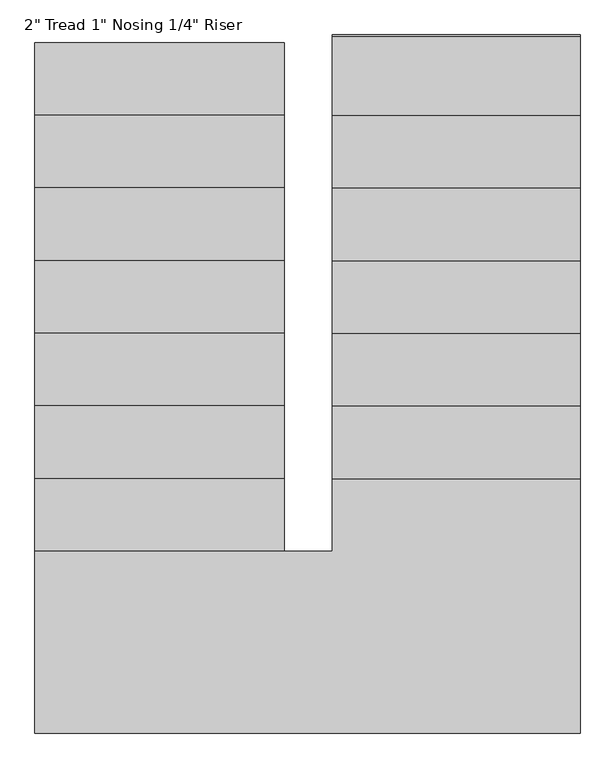
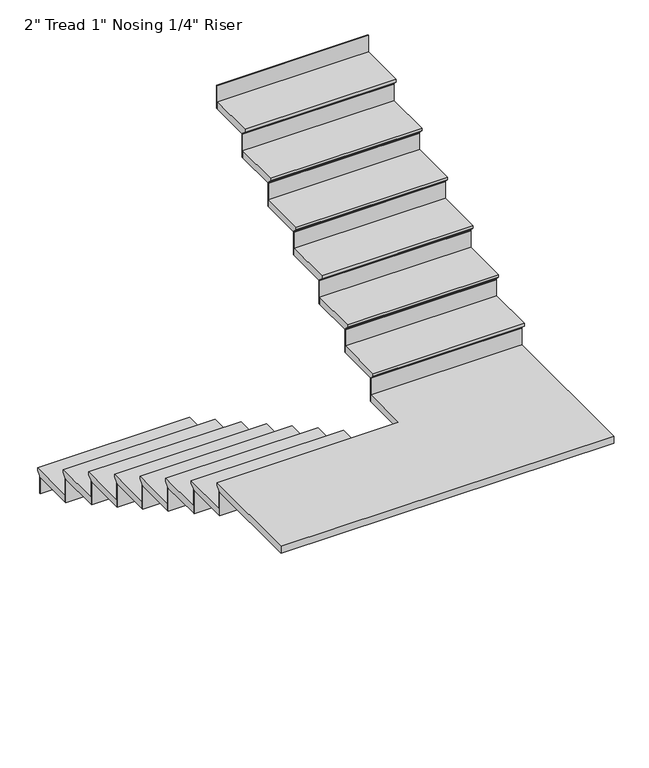
"""IFC4 building model written with IfcOpenShell, lengths in millimetres: stair flight geometry."""

from ifc_helpers import new_model, si_unit, origin, place, context, project, spatial, faceted_brep, source, transform, mapped, element, save


def stair_flight_d5b1d6b9(model_context):
    return source(origin(), model_context, "Body", "Brep", [
        faceted_brep([(-4232.280864, -3571.6080018, 3198.2833333), (-4232.280864, -3571.6080018, 3217.3333333), (-3187.6083919, -3571.6080018, 3217.3333333), (-3187.6083919, -3571.6080018, 3198.2833333), (-4232.280864, -3597.0080018, 3172.8833333), (-3187.6083919, -3597.0080018, 3172.8833333), (-4232.280864, -3901.8080018, 3217.3333333), (-3187.6083919, -3901.8080018, 3217.3333333), (-3187.6083919, -3597.0080018, 3166.5333333), (-3187.6083919, -3901.8080018, 3166.5333333), (-4232.280864, -3901.8080018, 3166.5333333), (-4232.280864, -3597.0080018, 3166.5333333)], [[[0, 1, 2, 3]], [[4, 0, 3, 5]], [[2, 1, 6, 7]], [[8, 9, 10, 11]], [[2, 7, 9, 8, 5, 3]], [[8, 11, 4, 5]], [[6, 1, 0, 4, 11, 10]], [[7, 6, 10, 9]]]),
        faceted_brep([(-4232.280864, -3597.0080018, 3166.5333333), (-4232.280864, -3597.0080018, 3048.0), (-4232.280864, -3603.3580018, 3048.0), (-4232.280864, -3603.3580018, 3166.5333333), (-3187.6083919, -3597.0080018, 3166.5333333), (-3187.6083919, -3603.3580018, 3166.5333333), (-3187.6083919, -3603.3580018, 3048.0), (-3187.6083919, -3597.0080018, 3048.0)], [[[0, 1, 2, 3]], [[4, 5, 6, 7]], [[1, 0, 4, 7]], [[2, 1, 7, 6]], [[3, 2, 6, 5]], [[0, 3, 5, 4]]]),
        faceted_brep([(-4232.280864, -3901.8080018, 3335.8666667), (-4232.280864, -3901.8080018, 3166.5333333), (-4232.280864, -3908.1580018, 3166.5333333), (-4232.280864, -3908.1580018, 3335.8666667), (-3187.6083919, -3901.8080018, 3335.8666667), (-3187.6083919, -3908.1580018, 3335.8666667), (-3187.6083919, -3908.1580018, 3166.5333333), (-3187.6083919, -3901.8080018, 3166.5333333)], [[[0, 1, 2, 3]], [[4, 5, 6, 7]], [[1, 0, 4, 7]], [[2, 1, 7, 6]], [[3, 2, 6, 5]], [[0, 3, 5, 4]]]),
        faceted_brep([(-3187.6083919, -3876.4080018, 3386.6666667), (-4232.280864, -3876.4080018, 3386.6666667), (-4232.280864, -4206.6080018, 3386.6666667), (-3187.6083919, -4206.6080018, 3386.6666667), (-3187.6083919, -3901.8080018, 3335.8666667), (-3187.6083919, -4206.6080018, 3335.8666667), (-4232.280864, -4206.6080018, 3335.8666667), (-4232.280864, -3901.8080018, 3335.8666667), (-3187.6083919, -3901.8080018, 3342.2166667), (-3187.6083919, -3876.4080018, 3367.6166667), (-4232.280864, -3901.8080018, 3342.2166667), (-4232.280864, -3876.4080018, 3367.6166667)], [[[0, 1, 2, 3]], [[4, 5, 6, 7]], [[0, 3, 5, 4, 8, 9]], [[4, 7, 10, 8]], [[2, 1, 11, 10, 7, 6]], [[3, 2, 6, 5]], [[11, 1, 0, 9]], [[10, 11, 9, 8]]]),
        faceted_brep([(-4232.280864, -4206.6080018, 3505.2), (-4232.280864, -4206.6080018, 3335.8666667), (-4232.280864, -4212.9580018, 3335.8666667), (-4232.280864, -4212.9580018, 3505.2), (-3187.6083919, -4206.6080018, 3505.2), (-3187.6083919, -4212.9580018, 3505.2), (-3187.6083919, -4212.9580018, 3335.8666667), (-3187.6083919, -4206.6080018, 3335.8666667)], [[[0, 1, 2, 3]], [[4, 5, 6, 7]], [[1, 0, 4, 7]], [[2, 1, 7, 6]], [[3, 2, 6, 5]], [[0, 3, 5, 4]]]),
        faceted_brep([(-3187.6083919, -4181.2080018, 3556.0), (-4232.280864, -4181.2080018, 3556.0), (-4232.280864, -4511.4080018, 3556.0), (-3187.6083919, -4511.4080018, 3556.0), (-3187.6083919, -4206.6080018, 3505.2), (-3187.6083919, -4511.4080018, 3505.2), (-4232.280864, -4511.4080018, 3505.2), (-4232.280864, -4206.6080018, 3505.2), (-3187.6083919, -4206.6080018, 3511.55), (-3187.6083919, -4181.2080018, 3536.95), (-4232.280864, -4206.6080018, 3511.55), (-4232.280864, -4181.2080018, 3536.95)], [[[0, 1, 2, 3]], [[4, 5, 6, 7]], [[0, 3, 5, 4, 8, 9]], [[4, 7, 10, 8]], [[2, 1, 11, 10, 7, 6]], [[3, 2, 6, 5]], [[11, 1, 0, 9]], [[10, 11, 9, 8]]]),
        faceted_brep([(-4232.280864, -4511.4080018, 3674.5333333), (-4232.280864, -4511.4080018, 3505.2), (-4232.280864, -4517.7580018, 3505.2), (-4232.280864, -4517.7580018, 3674.5333333), (-3187.6083919, -4511.4080018, 3674.5333333), (-3187.6083919, -4517.7580018, 3674.5333333), (-3187.6083919, -4517.7580018, 3505.2), (-3187.6083919, -4511.4080018, 3505.2)], [[[0, 1, 2, 3]], [[4, 5, 6, 7]], [[1, 0, 4, 7]], [[2, 1, 7, 6]], [[3, 2, 6, 5]], [[0, 3, 5, 4]]]),
        faceted_brep([(-3187.6083919, -4486.0080018, 3725.3333333), (-4232.280864, -4486.0080018, 3725.3333333), (-4232.280864, -4816.2080018, 3725.3333333), (-3187.6083919, -4816.2080018, 3725.3333333), (-3187.6083919, -4511.4080018, 3674.5333333), (-3187.6083919, -4816.2080018, 3674.5333333), (-4232.280864, -4816.2080018, 3674.5333333), (-4232.280864, -4511.4080018, 3674.5333333), (-3187.6083919, -4511.4080018, 3680.8833333), (-3187.6083919, -4486.0080018, 3706.2833333), (-4232.280864, -4511.4080018, 3680.8833333), (-4232.280864, -4486.0080018, 3706.2833333)], [[[0, 1, 2, 3]], [[4, 5, 6, 7]], [[0, 3, 5, 4, 8, 9]], [[4, 7, 10, 8]], [[2, 1, 11, 10, 7, 6]], [[3, 2, 6, 5]], [[11, 1, 0, 9]], [[10, 11, 9, 8]]]),
        faceted_brep([(-4232.280864, -4816.2080018, 3843.8666667), (-4232.280864, -4816.2080018, 3674.5333333), (-4232.280864, -4822.5580018, 3674.5333333), (-4232.280864, -4822.5580018, 3843.8666667), (-3187.6083919, -4816.2080018, 3843.8666667), (-3187.6083919, -4822.5580018, 3843.8666667), (-3187.6083919, -4822.5580018, 3674.5333333), (-3187.6083919, -4816.2080018, 3674.5333333)], [[[0, 1, 2, 3]], [[4, 5, 6, 7]], [[1, 0, 4, 7]], [[2, 1, 7, 6]], [[3, 2, 6, 5]], [[0, 3, 5, 4]]]),
        faceted_brep([(-3187.6083919, -4790.8080018, 3894.6666667), (-4232.280864, -4790.8080018, 3894.6666667), (-4232.280864, -5121.0080018, 3894.6666667), (-3187.6083919, -5121.0080018, 3894.6666667), (-3187.6083919, -4816.2080018, 3843.8666667), (-3187.6083919, -5121.0080018, 3843.8666667), (-4232.280864, -5121.0080018, 3843.8666667), (-4232.280864, -4816.2080018, 3843.8666667), (-3187.6083919, -4816.2080018, 3850.2166667), (-3187.6083919, -4790.8080018, 3875.6166667), (-4232.280864, -4816.2080018, 3850.2166667), (-4232.280864, -4790.8080018, 3875.6166667)], [[[0, 1, 2, 3]], [[4, 5, 6, 7]], [[0, 3, 5, 4, 8, 9]], [[4, 7, 10, 8]], [[2, 1, 11, 10, 7, 6]], [[3, 2, 6, 5]], [[11, 1, 0, 9]], [[10, 11, 9, 8]]]),
        faceted_brep([(-4232.280864, -5121.0080018, 4013.2), (-4232.280864, -5121.0080018, 3843.8666667), (-4232.280864, -5127.3580018, 3843.8666667), (-4232.280864, -5127.3580018, 4013.2), (-3187.6083919, -5121.0080018, 4013.2), (-3187.6083919, -5127.3580018, 4013.2), (-3187.6083919, -5127.3580018, 3843.8666667), (-3187.6083919, -5121.0080018, 3843.8666667)], [[[0, 1, 2, 3]], [[4, 5, 6, 7]], [[1, 0, 4, 7]], [[2, 1, 7, 6]], [[3, 2, 6, 5]], [[0, 3, 5, 4]]]),
        faceted_brep([(-3187.6083919, -5095.6080018, 4064.0), (-4232.280864, -5095.6080018, 4064.0), (-4232.280864, -5425.8080018, 4064.0), (-3187.6083919, -5425.8080018, 4064.0), (-3187.6083919, -5121.0080018, 4013.2), (-3187.6083919, -5425.8080018, 4013.2), (-4232.280864, -5425.8080018, 4013.2), (-4232.280864, -5121.0080018, 4013.2), (-3187.6083919, -5121.0080018, 4019.55), (-3187.6083919, -5095.6080018, 4044.95), (-4232.280864, -5121.0080018, 4019.55), (-4232.280864, -5095.6080018, 4044.95)], [[[0, 1, 2, 3]], [[4, 5, 6, 7]], [[0, 3, 5, 4, 8, 9]], [[4, 7, 10, 8]], [[2, 1, 11, 10, 7, 6]], [[3, 2, 6, 5]], [[11, 1, 0, 9]], [[10, 11, 9, 8]]]),
        faceted_brep([(-4232.280864, -5425.8080018, 4182.5333333), (-4232.280864, -5425.8080018, 4013.2), (-4232.280864, -5432.1580018, 4013.2), (-4232.280864, -5432.1580018, 4182.5333333), (-3187.6083919, -5425.8080018, 4182.5333333), (-3187.6083919, -5432.1580018, 4182.5333333), (-3187.6083919, -5432.1580018, 4013.2), (-3187.6083919, -5425.8080018, 4013.2)], [[[0, 1, 2, 3]], [[4, 5, 6, 7]], [[1, 0, 4, 7]], [[2, 1, 7, 6]], [[3, 2, 6, 5]], [[0, 3, 5, 4]]]),
        faceted_brep([(-3187.6083919, -5400.4080018, 4233.3333333), (-4232.280864, -5400.4080018, 4233.3333333), (-4232.280864, -5730.6080018, 4233.3333333), (-3187.6083919, -5730.6080018, 4233.3333333), (-3187.6083919, -5425.8080018, 4182.5333333), (-3187.6083919, -5730.6080018, 4182.5333333), (-4232.280864, -5730.6080018, 4182.5333333), (-4232.280864, -5425.8080018, 4182.5333333), (-3187.6083919, -5425.8080018, 4188.8833333), (-3187.6083919, -5400.4080018, 4214.2833333), (-4232.280864, -5425.8080018, 4188.8833333), (-4232.280864, -5400.4080018, 4214.2833333)], [[[0, 1, 2, 3]], [[4, 5, 6, 7]], [[0, 3, 5, 4, 8, 9]], [[4, 7, 10, 8]], [[2, 1, 11, 10, 7, 6]], [[3, 2, 6, 5]], [[11, 1, 0, 9]], [[10, 11, 9, 8]]]),
        faceted_brep([(-4232.280864, -5730.6080018, 4351.8666667), (-4232.280864, -5730.6080018, 4182.5333333), (-4232.280864, -5736.9580018, 4182.5333333), (-4232.280864, -5736.9580018, 4351.8666667), (-3187.6083919, -5730.6080018, 4351.8666667), (-3187.6083919, -5736.9580018, 4351.8666667), (-3187.6083919, -5736.9580018, 4182.5333333), (-3187.6083919, -5730.6080018, 4182.5333333)], [[[0, 1, 2, 3]], [[4, 5, 6, 7]], [[1, 0, 4, 7]], [[2, 1, 7, 6]], [[3, 2, 6, 5]], [[0, 3, 5, 4]]]),
        faceted_brep([(-2984.4083919, -5375.0080018, 4402.6666667), (-2984.4083919, -5705.2080018, 4402.6666667), (-4232.280864, -5705.2080018, 4402.6666667), (-4232.280864, -6467.2080018, 4402.6666667), (-1946.280864, -6467.2080018, 4402.6666667), (-1946.280864, -5375.0080018, 4402.6666667), (-2984.4083919, -5705.2080018, 4351.8666667), (-2984.4083919, -5375.0080018, 4351.8666667), (-1946.280864, -5375.0080018, 4351.8666667), (-1946.280864, -6467.2080018, 4351.8666667), (-4232.280864, -6467.2080018, 4351.8666667), (-4232.280864, -5730.6080018, 4351.8666667), (-3187.6083919, -5730.6080018, 4351.8666667), (-3187.6083919, -5705.2080018, 4351.8666667), (-3187.6083919, -5705.2080018, 4383.6166667), (-4232.280864, -5705.2080018, 4383.6166667), (-3187.6083919, -5730.6080018, 4358.2166667), (-4232.280864, -5730.6080018, 4358.2166667)], [[[0, 1, 2, 3, 4, 5]], [[6, 7, 8, 9, 10, 11, 12, 13]], [[1, 0, 7, 6]], [[2, 1, 6, 13, 14, 15]], [[13, 12, 16, 14]], [[12, 11, 17, 16]], [[3, 2, 15, 17, 11, 10]], [[4, 3, 10, 9]], [[5, 4, 9, 8]], [[0, 5, 8, 7]], [[17, 15, 14, 16]]]),
        faceted_brep([(-1946.280864, -5375.0080018, 4521.2), (-1946.280864, -5375.0080018, 4351.8666667), (-1946.280864, -5368.6580018, 4351.8666667), (-1946.280864, -5368.6580018, 4521.2), (-2984.4083919, -5375.0080018, 4521.2), (-2984.4083919, -5368.6580018, 4521.2), (-2984.4083919, -5368.6580018, 4351.8666667), (-2984.4083919, -5375.0080018, 4351.8666667)], [[[0, 1, 2, 3]], [[4, 5, 6, 7]], [[1, 0, 4, 7]], [[2, 1, 7, 6]], [[3, 2, 6, 5]], [[0, 3, 5, 4]]]),
        faceted_brep([(-2984.4083919, -5400.4080018, 4572.0), (-1946.280864, -5400.4080018, 4572.0), (-1946.280864, -5070.2080018, 4572.0), (-2984.4083919, -5070.2080018, 4572.0), (-2984.4083919, -5375.0080018, 4521.2), (-2984.4083919, -5070.2080018, 4521.2), (-1946.280864, -5070.2080018, 4521.2), (-1946.280864, -5375.0080018, 4521.2), (-2984.4083919, -5375.0080018, 4527.55), (-2984.4083919, -5400.4080018, 4552.95), (-1946.280864, -5375.0080018, 4527.55), (-1946.280864, -5400.4080018, 4552.95)], [[[0, 1, 2, 3]], [[4, 5, 6, 7]], [[0, 3, 5, 4, 8, 9]], [[4, 7, 10, 8]], [[2, 1, 11, 10, 7, 6]], [[3, 2, 6, 5]], [[11, 1, 0, 9]], [[10, 11, 9, 8]]]),
        faceted_brep([(-1946.280864, -5070.2080018, 4690.5333333), (-1946.280864, -5070.2080018, 4521.2), (-1946.280864, -5063.8580018, 4521.2), (-1946.280864, -5063.8580018, 4690.5333333), (-2984.4083919, -5070.2080018, 4690.5333333), (-2984.4083919, -5063.8580018, 4690.5333333), (-2984.4083919, -5063.8580018, 4521.2), (-2984.4083919, -5070.2080018, 4521.2)], [[[0, 1, 2, 3]], [[4, 5, 6, 7]], [[1, 0, 4, 7]], [[2, 1, 7, 6]], [[3, 2, 6, 5]], [[0, 3, 5, 4]]]),
        faceted_brep([(-2984.4083919, -5095.6080018, 4741.3333333), (-1946.280864, -5095.6080018, 4741.3333333), (-1946.280864, -4765.4080018, 4741.3333333), (-2984.4083919, -4765.4080018, 4741.3333333), (-2984.4083919, -5070.2080018, 4690.5333333), (-2984.4083919, -4765.4080018, 4690.5333333), (-1946.280864, -4765.4080018, 4690.5333333), (-1946.280864, -5070.2080018, 4690.5333333), (-2984.4083919, -5070.2080018, 4696.8833333), (-2984.4083919, -5095.6080018, 4722.2833333), (-1946.280864, -5070.2080018, 4696.8833333), (-1946.280864, -5095.6080018, 4722.2833333)], [[[0, 1, 2, 3]], [[4, 5, 6, 7]], [[0, 3, 5, 4, 8, 9]], [[4, 7, 10, 8]], [[2, 1, 11, 10, 7, 6]], [[3, 2, 6, 5]], [[11, 1, 0, 9]], [[10, 11, 9, 8]]]),
        faceted_brep([(-1946.280864, -4765.4080018, 4859.8666667), (-1946.280864, -4765.4080018, 4690.5333333), (-1946.280864, -4759.0580018, 4690.5333333), (-1946.280864, -4759.0580018, 4859.8666667), (-2984.4083919, -4765.4080018, 4859.8666667), (-2984.4083919, -4759.0580018, 4859.8666667), (-2984.4083919, -4759.0580018, 4690.5333333), (-2984.4083919, -4765.4080018, 4690.5333333)], [[[0, 1, 2, 3]], [[4, 5, 6, 7]], [[1, 0, 4, 7]], [[2, 1, 7, 6]], [[3, 2, 6, 5]], [[0, 3, 5, 4]]]),
        faceted_brep([(-2984.4083919, -4790.8080018, 4910.6666667), (-1946.280864, -4790.8080018, 4910.6666667), (-1946.280864, -4460.6080018, 4910.6666667), (-2984.4083919, -4460.6080018, 4910.6666667), (-2984.4083919, -4765.4080018, 4859.8666667), (-2984.4083919, -4460.6080018, 4859.8666667), (-1946.280864, -4460.6080018, 4859.8666667), (-1946.280864, -4765.4080018, 4859.8666667), (-2984.4083919, -4765.4080018, 4866.2166667), (-2984.4083919, -4790.8080018, 4891.6166667), (-1946.280864, -4765.4080018, 4866.2166667), (-1946.280864, -4790.8080018, 4891.6166667)], [[[0, 1, 2, 3]], [[4, 5, 6, 7]], [[0, 3, 5, 4, 8, 9]], [[4, 7, 10, 8]], [[2, 1, 11, 10, 7, 6]], [[3, 2, 6, 5]], [[11, 1, 0, 9]], [[10, 11, 9, 8]]]),
        faceted_brep([(-1946.280864, -4460.6080018, 5029.2), (-1946.280864, -4460.6080018, 4859.8666667), (-1946.280864, -4454.2580018, 4859.8666667), (-1946.280864, -4454.2580018, 5029.2), (-2984.4083919, -4460.6080018, 5029.2), (-2984.4083919, -4454.2580018, 5029.2), (-2984.4083919, -4454.2580018, 4859.8666667), (-2984.4083919, -4460.6080018, 4859.8666667)], [[[0, 1, 2, 3]], [[4, 5, 6, 7]], [[1, 0, 4, 7]], [[2, 1, 7, 6]], [[3, 2, 6, 5]], [[0, 3, 5, 4]]]),
        faceted_brep([(-2984.4083919, -4486.0080018, 5080.0), (-1946.280864, -4486.0080018, 5080.0), (-1946.280864, -4155.8080018, 5080.0), (-2984.4083919, -4155.8080018, 5080.0), (-2984.4083919, -4460.6080018, 5029.2), (-2984.4083919, -4155.8080018, 5029.2), (-1946.280864, -4155.8080018, 5029.2), (-1946.280864, -4460.6080018, 5029.2), (-2984.4083919, -4460.6080018, 5035.55), (-2984.4083919, -4486.0080018, 5060.95), (-1946.280864, -4460.6080018, 5035.55), (-1946.280864, -4486.0080018, 5060.95)], [[[0, 1, 2, 3]], [[4, 5, 6, 7]], [[0, 3, 5, 4, 8, 9]], [[4, 7, 10, 8]], [[2, 1, 11, 10, 7, 6]], [[3, 2, 6, 5]], [[11, 1, 0, 9]], [[10, 11, 9, 8]]]),
        faceted_brep([(-1946.280864, -4155.8080018, 5198.5333333), (-1946.280864, -4155.8080018, 5029.2), (-1946.280864, -4149.4580018, 5029.2), (-1946.280864, -4149.4580018, 5198.5333333), (-2984.4083919, -4155.8080018, 5198.5333333), (-2984.4083919, -4149.4580018, 5198.5333333), (-2984.4083919, -4149.4580018, 5029.2), (-2984.4083919, -4155.8080018, 5029.2)], [[[0, 1, 2, 3]], [[4, 5, 6, 7]], [[1, 0, 4, 7]], [[2, 1, 7, 6]], [[3, 2, 6, 5]], [[0, 3, 5, 4]]]),
        faceted_brep([(-2984.4083919, -4181.2080018, 5249.3333333), (-1946.280864, -4181.2080018, 5249.3333333), (-1946.280864, -3851.0080018, 5249.3333333), (-2984.4083919, -3851.0080018, 5249.3333333), (-2984.4083919, -4155.8080018, 5198.5333333), (-2984.4083919, -3851.0080018, 5198.5333333), (-1946.280864, -3851.0080018, 5198.5333333), (-1946.280864, -4155.8080018, 5198.5333333), (-2984.4083919, -4155.8080018, 5204.8833333), (-2984.4083919, -4181.2080018, 5230.2833333), (-1946.280864, -4155.8080018, 5204.8833333), (-1946.280864, -4181.2080018, 5230.2833333)], [[[0, 1, 2, 3]], [[4, 5, 6, 7]], [[0, 3, 5, 4, 8, 9]], [[4, 7, 10, 8]], [[2, 1, 11, 10, 7, 6]], [[3, 2, 6, 5]], [[11, 1, 0, 9]], [[10, 11, 9, 8]]]),
        faceted_brep([(-1946.280864, -3851.0080018, 5367.8666667), (-1946.280864, -3851.0080018, 5198.5333333), (-1946.280864, -3844.6580018, 5198.5333333), (-1946.280864, -3844.6580018, 5367.8666667), (-2984.4083919, -3851.0080018, 5367.8666667), (-2984.4083919, -3844.6580018, 5367.8666667), (-2984.4083919, -3844.6580018, 5198.5333333), (-2984.4083919, -3851.0080018, 5198.5333333)], [[[0, 1, 2, 3]], [[4, 5, 6, 7]], [[1, 0, 4, 7]], [[2, 1, 7, 6]], [[3, 2, 6, 5]], [[0, 3, 5, 4]]]),
        faceted_brep([(-1946.280864, -3546.2080018, 5537.2), (-1946.280864, -3546.2080018, 5367.8666667), (-1946.280864, -3539.8580018, 5367.8666667), (-1946.280864, -3539.8580018, 5537.2), (-2984.4083919, -3546.2080018, 5537.2), (-2984.4083919, -3539.8580018, 5537.2), (-2984.4083919, -3539.8580018, 5367.8666667), (-2984.4083919, -3546.2080018, 5367.8666667)], [[[0, 1, 2, 3]], [[4, 5, 6, 7]], [[1, 0, 4, 7]], [[2, 1, 7, 6]], [[3, 2, 6, 5]], [[0, 3, 5, 4]]]),
        faceted_brep([(-2984.4083919, -3876.4080018, 5418.6666667), (-1946.280864, -3876.4080018, 5418.6666667), (-1946.280864, -3546.2080018, 5418.6666667), (-2984.4083919, -3546.2080018, 5418.6666667), (-2984.4083919, -3851.0080018, 5367.8666667), (-2984.4083919, -3546.2080018, 5367.8666667), (-1946.280864, -3546.2080018, 5367.8666667), (-1946.280864, -3851.0080018, 5367.8666667), (-2984.4083919, -3851.0080018, 5374.2166667), (-2984.4083919, -3876.4080018, 5399.6166667), (-1946.280864, -3851.0080018, 5374.2166667), (-1946.280864, -3876.4080018, 5399.6166667)], [[[0, 1, 2, 3]], [[4, 5, 6, 7]], [[0, 3, 5, 4, 8, 9]], [[4, 7, 10, 8]], [[2, 1, 11, 10, 7, 6]], [[3, 2, 6, 5]], [[11, 1, 0, 9]], [[10, 11, 9, 8]]]),
    ])


if __name__ == "__main__":
    model = new_model("IFC4")
    model_context = context("Model", 3, world=origin())
    ifc_project = project(units=[si_unit("LENGTHUNIT", "METRE", prefix="MILLI")], contexts=[model_context])
    site = spatial("IfcSite", under=ifc_project)
    building = spatial("IfcBuilding", under=site)
    placement = place(None, origin())
    stair_flight_shape = stair_flight_d5b1d6b9(model_context)
    element("IfcStairFlight", 1, ObjectType="2\" Tread 1\" Nosing 1/4\" Riser", at=placement, inside=building, context=model_context, shape_type="MappedRepresentation", body=[
        mapped(stair_flight_shape, transform((0.0, 0.0, 0.0), x_axis=(1.0, 0.0, 0.0), y_axis=(0.0, 1.0, 0.0), z_axis=(0.0, 0.0, 1.0))),
    ])
    save(model, "model.ifc")
